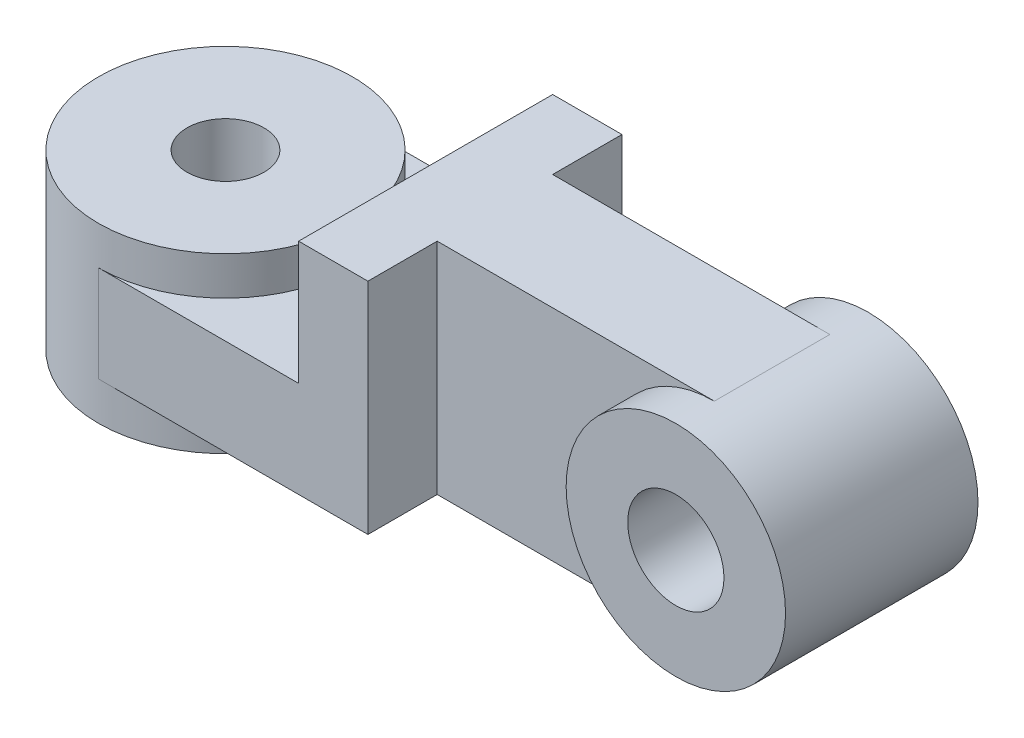
ISO-10303-21;
HEADER;
FILE_DESCRIPTION(('STEP AP214'),'2;1');
FILE_NAME('part.step','',(''),(''),'','','');
FILE_SCHEMA(('AUTOMOTIVE_DESIGN { 1 0 10303 214 1 1 1 1 }'));
ENDSEC;
DATA;
#1=APPLICATION_CONTEXT('core data for automotive mechanical design processes');
#2=APPLICATION_PROTOCOL_DEFINITION('international standard','automotive_design',2000,#1);
#3=PRODUCT_CONTEXT('',#1,'mechanical');
#4=PRODUCT('Part','Part','',(#3));
#5=PRODUCT_RELATED_PRODUCT_CATEGORY('part','',(#4));
#6=PRODUCT_DEFINITION_FORMATION('','',#4);
#7=PRODUCT_DEFINITION_CONTEXT('part definition',#1,'design');
#8=PRODUCT_DEFINITION('design','',#6,#7);
#9=PRODUCT_DEFINITION_SHAPE('','',#8);
#10=(LENGTH_UNIT() NAMED_UNIT(*) SI_UNIT(.MILLI.,.METRE.));
#11=(NAMED_UNIT(*) PLANE_ANGLE_UNIT() SI_UNIT($,.RADIAN.));
#12=(NAMED_UNIT(*) SI_UNIT($,.STERADIAN.) SOLID_ANGLE_UNIT());
#13=UNCERTAINTY_MEASURE_WITH_UNIT(LENGTH_MEASURE(1.E-05),#10,'distance_accuracy_value','');
#14=(GEOMETRIC_REPRESENTATION_CONTEXT(3) GLOBAL_UNCERTAINTY_ASSIGNED_CONTEXT((#13)) GLOBAL_UNIT_ASSIGNED_CONTEXT((#10,
#11,#12)) REPRESENTATION_CONTEXT('',''));
#15=CARTESIAN_POINT('',(0.,0.,0.));
#16=DIRECTION('',(0.,0.,1.));
#17=DIRECTION('',(1.,0.,0.));
#18=AXIS2_PLACEMENT_3D('',#15,#16,#17);
#19=CARTESIAN_POINT('',(70000.,12500.,-33000.));
#20=DIRECTION('',(-1.,0.,0.));
#21=DIRECTION('',(0.,0.,1.));
#22=AXIS2_PLACEMENT_3D('',#19,#20,#21);
#23=PLANE('',#22);
#24=DIRECTION('',(0.,1.,0.));
#25=VECTOR('',#24,1.);
#26=CARTESIAN_POINT('',(70000.,-12500.,-15000.));
#27=LINE('',#26,#25);
#28=CARTESIAN_POINT('',(70000.,-12500.,-15000.));
#29=VERTEX_POINT('',#28);
#30=CARTESIAN_POINT('',(70000.,44500.,-15000.));
#31=VERTEX_POINT('',#30);
#32=EDGE_CURVE('E152',#29,#31,#27,.T.);
#33=ORIENTED_EDGE('',*,*,#32,.F.);
#34=DIRECTION('',(0.,0.,-1.));
#35=VECTOR('',#34,1.);
#36=CARTESIAN_POINT('',(70000.,-12500.,-33000.));
#37=LINE('',#36,#35);
#38=CARTESIAN_POINT('',(70000.,-12500.,-33000.));
#39=VERTEX_POINT('',#38);
#40=EDGE_CURVE('E189',#29,#39,#37,.T.);
#41=ORIENTED_EDGE('',*,*,#40,.T.);
#42=DIRECTION('',(0.,-1.,0.));
#43=VECTOR('',#42,1.);
#44=CARTESIAN_POINT('',(70000.,12500.,-33000.));
#45=LINE('',#44,#43);
#46=CARTESIAN_POINT('',(70000.,44500.,-33000.));
#47=VERTEX_POINT('',#46);
#48=EDGE_CURVE('E191',#47,#39,#45,.T.);
#49=ORIENTED_EDGE('',*,*,#48,.F.);
#50=DIRECTION('',(0.,0.,-1.));
#51=VECTOR('',#50,1.);
#52=CARTESIAN_POINT('',(70000.,44500.,33000.));
#53=LINE('',#52,#51);
#54=EDGE_CURVE('E163',#31,#47,#53,.T.);
#55=ORIENTED_EDGE('',*,*,#54,.F.);
#56=EDGE_LOOP('',(#33,#41,#49,#55));
#57=FACE_BOUND('',#56,.T.);
#58=ADVANCED_FACE('F50',(#57),#23,.F.);
#59=CARTESIAN_POINT('',(0.,12500.,0.));
#60=DIRECTION('',(0.,1.,0.));
#61=DIRECTION('',(0.,0.,1.));
#62=AXIS2_PLACEMENT_3D('',#59,#60,#61);
#63=PLANE('',#62);
#64=DIRECTION('',(1.,0.,0.));
#65=VECTOR('',#64,1.);
#66=CARTESIAN_POINT('',(0.,12500.,33000.));
#67=LINE('',#66,#65);
#68=CARTESIAN_POINT('',(0.,12500.,33000.));
#69=VERTEX_POINT('',#68);
#70=CARTESIAN_POINT('',(52000.,12500.,33000.));
#71=VERTEX_POINT('',#70);
#72=EDGE_CURVE('E177',#69,#71,#67,.T.);
#73=ORIENTED_EDGE('',*,*,#72,.T.);
#74=DIRECTION('',(0.,0.,1.));
#75=VECTOR('',#74,1.);
#76=CARTESIAN_POINT('',(52000.,12500.,33000.));
#77=LINE('',#76,#75);
#78=CARTESIAN_POINT('',(52000.,12500.,-33000.));
#79=VERTEX_POINT('',#78);
#80=EDGE_CURVE('E67',#79,#71,#77,.T.);
#81=ORIENTED_EDGE('',*,*,#80,.F.);
#82=DIRECTION('',(-1.,0.,0.));
#83=VECTOR('',#82,1.);
#84=CARTESIAN_POINT('',(0.,12500.,-33000.));
#85=LINE('',#84,#83);
#86=CARTESIAN_POINT('',(-2.00982088115E-11,12500.,-33000.));
#87=VERTEX_POINT('',#86);
#88=EDGE_CURVE('E185',#79,#87,#85,.T.);
#89=ORIENTED_EDGE('',*,*,#88,.T.);
#90=CARTESIAN_POINT('',(0.,12500.,0.));
#91=DIRECTION('',(0.,-1.,0.));
#92=DIRECTION('',(0.,0.,1.));
#93=AXIS2_PLACEMENT_3D('',#90,#91,#92);
#94=CIRCLE('',#93,33000.);
#95=EDGE_CURVE('E176',#87,#69,#94,.T.);
#96=ORIENTED_EDGE('',*,*,#95,.T.);
#97=EDGE_LOOP('',(#73,#81,#89,#96));
#98=FACE_BOUND('',#97,.T.);
#99=ADVANCED_FACE('F233',(#98),#63,.T.);
#100=CARTESIAN_POINT('',(0.,22500.,0.));
#101=DIRECTION('',(0.,-1.,0.));
#102=DIRECTION('',(0.,0.,-1.));
#103=AXIS2_PLACEMENT_3D('',#100,#101,#102);
#104=CYLINDRICAL_SURFACE('',#103,33000.);
#105=DIRECTION('',(0.,-1.,0.));
#106=VECTOR('',#105,1.);
#107=CARTESIAN_POINT('',(0.,12500.,33000.));
#108=LINE('',#107,#106);
#109=CARTESIAN_POINT('',(0.,-12500.,33000.));
#110=VERTEX_POINT('',#109);
#111=EDGE_CURVE('E199',#69,#110,#108,.T.);
#112=ORIENTED_EDGE('',*,*,#111,.F.);
#113=ORIENTED_EDGE('',*,*,#95,.F.);
#114=DIRECTION('',(0.,-1.,0.));
#115=VECTOR('',#114,1.);
#116=CARTESIAN_POINT('',(0.,12500.,-33000.));
#117=LINE('',#116,#115);
#118=CARTESIAN_POINT('',(0.,-12500.,-33000.));
#119=VERTEX_POINT('',#118);
#120=EDGE_CURVE('E183',#87,#119,#117,.T.);
#121=ORIENTED_EDGE('',*,*,#120,.T.);
#122=CARTESIAN_POINT('',(0.,-12500.,0.));
#123=DIRECTION('',(0.,-1.,0.));
#124=DIRECTION('',(0.,0.,1.));
#125=AXIS2_PLACEMENT_3D('',#122,#123,#124);
#126=CIRCLE('',#125,33000.);
#127=EDGE_CURVE('E174',#119,#110,#126,.T.);
#128=ORIENTED_EDGE('',*,*,#127,.T.);
#129=EDGE_LOOP('',(#112,#113,#121,#128));
#130=FACE_BOUND('',#129,.T.);
#131=CARTESIAN_POINT('',(0.,22500.,0.));
#132=DIRECTION('',(0.,1.,0.));
#133=DIRECTION('',(0.,0.,1.));
#134=AXIS2_PLACEMENT_3D('',#131,#132,#133);
#135=CIRCLE('',#134,33000.);
#136=CARTESIAN_POINT('',(0.,22500.,33000.));
#137=VERTEX_POINT('',#136);
#138=EDGE_CURVE('E54',#137,#137,#135,.T.);
#139=ORIENTED_EDGE('',*,*,#138,.F.);
#140=EDGE_LOOP('',(#139));
#141=FACE_BOUND('',#140,.T.);
#142=CARTESIAN_POINT('',(0.,-22500.,0.));
#143=DIRECTION('',(0.,1.,0.));
#144=DIRECTION('',(0.,0.,1.));
#145=AXIS2_PLACEMENT_3D('',#142,#143,#144);
#146=CIRCLE('',#145,33000.);
#147=CARTESIAN_POINT('',(0.,-22500.,33000.));
#148=VERTEX_POINT('',#147);
#149=EDGE_CURVE('E210',#148,#148,#146,.T.);
#150=ORIENTED_EDGE('',*,*,#149,.T.);
#151=EDGE_LOOP('',(#150));
#152=FACE_BOUND('',#151,.T.);
#153=ADVANCED_FACE('F47',(#130,#141,#152),#104,.T.);
#154=CARTESIAN_POINT('',(0.,22500.,0.));
#155=DIRECTION('',(0.,1.,0.));
#156=DIRECTION('',(0.,0.,1.));
#157=AXIS2_PLACEMENT_3D('',#154,#155,#156);
#158=PLANE('',#157);
#159=CARTESIAN_POINT('',(0.,22500.,0.));
#160=DIRECTION('',(0.,1.,0.));
#161=DIRECTION('',(0.,0.,1.));
#162=AXIS2_PLACEMENT_3D('',#159,#160,#161);
#163=CIRCLE('',#162,10000.);
#164=CARTESIAN_POINT('',(0.,22500.,10000.));
#165=VERTEX_POINT('',#164);
#166=EDGE_CURVE('E203',#165,#165,#163,.T.);
#167=ORIENTED_EDGE('',*,*,#166,.F.);
#168=EDGE_LOOP('',(#167));
#169=FACE_BOUND('',#168,.T.);
#170=ORIENTED_EDGE('',*,*,#138,.T.);
#171=EDGE_LOOP('',(#170));
#172=FACE_BOUND('',#171,.T.);
#173=ADVANCED_FACE('F218',(#169,#172),#158,.T.);
#174=CARTESIAN_POINT('',(0.,-22500.,0.));
#175=DIRECTION('',(0.,1.,0.));
#176=DIRECTION('',(0.,0.,1.));
#177=AXIS2_PLACEMENT_3D('',#174,#175,#176);
#178=PLANE('',#177);
#179=CARTESIAN_POINT('',(0.,-22500.,0.));
#180=DIRECTION('',(0.,1.,0.));
#181=DIRECTION('',(0.,0.,1.));
#182=AXIS2_PLACEMENT_3D('',#179,#180,#181);
#183=CIRCLE('',#182,10000.);
#184=CARTESIAN_POINT('',(0.,-22500.,10000.));
#185=VERTEX_POINT('',#184);
#186=EDGE_CURVE('E202',#185,#185,#183,.T.);
#187=ORIENTED_EDGE('',*,*,#186,.T.);
#188=EDGE_LOOP('',(#187));
#189=FACE_BOUND('',#188,.T.);
#190=ORIENTED_EDGE('',*,*,#149,.F.);
#191=EDGE_LOOP('',(#190));
#192=FACE_BOUND('',#191,.T.);
#193=ADVANCED_FACE('F213',(#189,#192),#178,.F.);
#194=CARTESIAN_POINT('',(0.,-22500.,0.));
#195=DIRECTION('',(0.,1.,0.));
#196=DIRECTION('',(0.,0.,1.));
#197=AXIS2_PLACEMENT_3D('',#194,#195,#196);
#198=CYLINDRICAL_SURFACE('',#197,10000.);
#199=ORIENTED_EDGE('',*,*,#186,.F.);
#200=EDGE_LOOP('',(#199));
#201=FACE_BOUND('',#200,.T.);
#202=ORIENTED_EDGE('',*,*,#166,.T.);
#203=EDGE_LOOP('',(#202));
#204=FACE_BOUND('',#203,.T.);
#205=ADVANCED_FACE('F220',(#201,#204),#198,.F.);
#206=CARTESIAN_POINT('',(0.,12500.,33000.));
#207=DIRECTION('',(0.,0.,-1.));
#208=DIRECTION('',(-1.,0.,0.));
#209=AXIS2_PLACEMENT_3D('',#206,#207,#208);
#210=PLANE('',#209);
#211=DIRECTION('',(1.,0.,0.));
#212=VECTOR('',#211,1.);
#213=CARTESIAN_POINT('',(0.,-12500.,33000.));
#214=LINE('',#213,#212);
#215=CARTESIAN_POINT('',(70000.,-12500.,33000.));
#216=VERTEX_POINT('',#215);
#217=EDGE_CURVE('E187',#110,#216,#214,.T.);
#218=ORIENTED_EDGE('',*,*,#217,.T.);
#219=DIRECTION('',(0.,-1.,0.));
#220=VECTOR('',#219,1.);
#221=CARTESIAN_POINT('',(70000.,12500.,33000.));
#222=LINE('',#221,#220);
#223=CARTESIAN_POINT('',(70000.,44500.,33000.));
#224=VERTEX_POINT('',#223);
#225=EDGE_CURVE('E200',#224,#216,#222,.T.);
#226=ORIENTED_EDGE('',*,*,#225,.F.);
#227=DIRECTION('',(1.,0.,0.));
#228=VECTOR('',#227,1.);
#229=CARTESIAN_POINT('',(70000.,44500.,33000.));
#230=LINE('',#229,#228);
#231=CARTESIAN_POINT('',(52000.,44500.,33000.));
#232=VERTEX_POINT('',#231);
#233=EDGE_CURVE('E164',#232,#224,#230,.T.);
#234=ORIENTED_EDGE('',*,*,#233,.F.);
#235=DIRECTION('',(0.,-1.,0.));
#236=VECTOR('',#235,1.);
#237=CARTESIAN_POINT('',(52000.,44500.,33000.));
#238=LINE('',#237,#236);
#239=EDGE_CURVE('E166',#232,#71,#238,.T.);
#240=ORIENTED_EDGE('',*,*,#239,.T.);
#241=ORIENTED_EDGE('',*,*,#72,.F.);
#242=ORIENTED_EDGE('',*,*,#111,.T.);
#243=EDGE_LOOP('',(#218,#226,#234,#240,#241,#242));
#244=FACE_BOUND('',#243,.T.);
#245=ADVANCED_FACE('F222',(#244),#210,.F.);
#246=CARTESIAN_POINT('',(70000.,-12500.,15000.));
#247=VERTEX_POINT('',#246);
#248=EDGE_CURVE('E186',#216,#247,#37,.T.);
#249=ORIENTED_EDGE('',*,*,#248,.T.);
#250=DIRECTION('',(0.,1.,0.));
#251=VECTOR('',#250,1.);
#252=CARTESIAN_POINT('',(70000.,-12500.,15000.));
#253=LINE('',#252,#251);
#254=CARTESIAN_POINT('',(70000.,44500.,15000.));
#255=VERTEX_POINT('',#254);
#256=EDGE_CURVE('E145',#247,#255,#253,.T.);
#257=ORIENTED_EDGE('',*,*,#256,.T.);
#258=EDGE_CURVE('E160',#224,#255,#53,.T.);
#259=ORIENTED_EDGE('',*,*,#258,.F.);
#260=ORIENTED_EDGE('',*,*,#225,.T.);
#261=EDGE_LOOP('',(#249,#257,#259,#260));
#262=FACE_BOUND('',#261,.T.);
#263=ADVANCED_FACE('F234',(#262),#23,.F.);
#264=CARTESIAN_POINT('',(0.,12500.,-33000.));
#265=DIRECTION('',(0.,0.,1.));
#266=DIRECTION('',(1.,0.,0.));
#267=AXIS2_PLACEMENT_3D('',#264,#265,#266);
#268=PLANE('',#267);
#269=DIRECTION('',(-1.,0.,0.));
#270=VECTOR('',#269,1.);
#271=CARTESIAN_POINT('',(0.,-12500.,-33000.));
#272=LINE('',#271,#270);
#273=EDGE_CURVE('E179',#39,#119,#272,.T.);
#274=ORIENTED_EDGE('',*,*,#273,.T.);
#275=ORIENTED_EDGE('',*,*,#120,.F.);
#276=ORIENTED_EDGE('',*,*,#88,.F.);
#277=DIRECTION('',(0.,-1.,0.));
#278=VECTOR('',#277,1.);
#279=CARTESIAN_POINT('',(52000.,44500.,-33000.));
#280=LINE('',#279,#278);
#281=CARTESIAN_POINT('',(52000.,44500.,-33000.));
#282=VERTEX_POINT('',#281);
#283=EDGE_CURVE('E175',#282,#79,#280,.T.);
#284=ORIENTED_EDGE('',*,*,#283,.F.);
#285=DIRECTION('',(-1.,0.,0.));
#286=VECTOR('',#285,1.);
#287=CARTESIAN_POINT('',(70000.,44500.,-33000.));
#288=LINE('',#287,#286);
#289=EDGE_CURVE('E159',#47,#282,#288,.T.);
#290=ORIENTED_EDGE('',*,*,#289,.F.);
#291=ORIENTED_EDGE('',*,*,#48,.T.);
#292=EDGE_LOOP('',(#274,#275,#276,#284,#290,#291));
#293=FACE_BOUND('',#292,.T.);
#294=ADVANCED_FACE('F242',(#293),#268,.F.);
#295=CARTESIAN_POINT('',(0.,-12500.,0.));
#296=DIRECTION('',(0.,1.,0.));
#297=DIRECTION('',(0.,0.,1.));
#298=AXIS2_PLACEMENT_3D('',#295,#296,#297);
#299=PLANE('',#298);
#300=ORIENTED_EDGE('',*,*,#127,.F.);
#301=ORIENTED_EDGE('',*,*,#273,.F.);
#302=ORIENTED_EDGE('',*,*,#40,.F.);
#303=DIRECTION('',(-1.,0.,0.));
#304=VECTOR('',#303,1.);
#305=CARTESIAN_POINT('',(70000.,-12500.,-15000.));
#306=LINE('',#305,#304);
#307=CARTESIAN_POINT('',(142000.,-12500.,-15000.));
#308=VERTEX_POINT('',#307);
#309=EDGE_CURVE('E137',#308,#29,#306,.T.);
#310=ORIENTED_EDGE('',*,*,#309,.F.);
#311=DIRECTION('',(0.,0.,-1.));
#312=VECTOR('',#311,1.);
#313=CARTESIAN_POINT('',(142000.,-12500.,-15000.));
#314=LINE('',#313,#312);
#315=CARTESIAN_POINT('',(142000.,-12500.,15000.));
#316=VERTEX_POINT('',#315);
#317=EDGE_CURVE('E123',#316,#308,#314,.T.);
#318=ORIENTED_EDGE('',*,*,#317,.F.);
#319=DIRECTION('',(1.,0.,0.));
#320=VECTOR('',#319,1.);
#321=CARTESIAN_POINT('',(70000.,-12500.,15000.));
#322=LINE('',#321,#320);
#323=EDGE_CURVE('E136',#247,#316,#322,.T.);
#324=ORIENTED_EDGE('',*,*,#323,.F.);
#325=ORIENTED_EDGE('',*,*,#248,.F.);
#326=ORIENTED_EDGE('',*,*,#217,.F.);
#327=EDGE_LOOP('',(#300,#301,#302,#310,#318,#324,#325,#326));
#328=FACE_BOUND('',#327,.T.);
#329=ADVANCED_FACE('F132',(#328),#299,.F.);
#330=CARTESIAN_POINT('',(52000.,44500.,33000.));
#331=DIRECTION('',(1.,0.,0.));
#332=DIRECTION('',(0.,0.,-1.));
#333=AXIS2_PLACEMENT_3D('',#330,#331,#332);
#334=PLANE('',#333);
#335=ORIENTED_EDGE('',*,*,#80,.T.);
#336=ORIENTED_EDGE('',*,*,#239,.F.);
#337=DIRECTION('',(0.,0.,1.));
#338=VECTOR('',#337,1.);
#339=CARTESIAN_POINT('',(52000.,44500.,33000.));
#340=LINE('',#339,#338);
#341=EDGE_CURVE('E161',#282,#232,#340,.T.);
#342=ORIENTED_EDGE('',*,*,#341,.F.);
#343=ORIENTED_EDGE('',*,*,#283,.T.);
#344=EDGE_LOOP('',(#335,#336,#342,#343));
#345=FACE_BOUND('',#344,.T.);
#346=ADVANCED_FACE('F271',(#345),#334,.F.);
#347=CARTESIAN_POINT('',(0.,44500.,0.));
#348=DIRECTION('',(0.,1.,0.));
#349=DIRECTION('',(0.,0.,1.));
#350=AXIS2_PLACEMENT_3D('',#347,#348,#349);
#351=PLANE('',#350);
#352=ORIENTED_EDGE('',*,*,#258,.T.);
#353=DIRECTION('',(1.,0.,0.));
#354=VECTOR('',#353,1.);
#355=CARTESIAN_POINT('',(70000.,44500.,15000.));
#356=LINE('',#355,#354);
#357=CARTESIAN_POINT('',(142000.,44500.,15000.));
#358=VERTEX_POINT('',#357);
#359=EDGE_CURVE('E62',#255,#358,#356,.T.);
#360=ORIENTED_EDGE('',*,*,#359,.T.);
#361=DIRECTION('',(0.,0.,-1.));
#362=VECTOR('',#361,1.);
#363=CARTESIAN_POINT('',(142000.,44500.,-15000.));
#364=LINE('',#363,#362);
#365=CARTESIAN_POINT('',(142000.,44500.,-15000.));
#366=VERTEX_POINT('',#365);
#367=EDGE_CURVE('E129',#358,#366,#364,.T.);
#368=ORIENTED_EDGE('',*,*,#367,.T.);
#369=DIRECTION('',(-1.,0.,0.));
#370=VECTOR('',#369,1.);
#371=CARTESIAN_POINT('',(70000.,44500.,-15000.));
#372=LINE('',#371,#370);
#373=EDGE_CURVE('E141',#366,#31,#372,.T.);
#374=ORIENTED_EDGE('',*,*,#373,.T.);
#375=ORIENTED_EDGE('',*,*,#54,.T.);
#376=ORIENTED_EDGE('',*,*,#289,.T.);
#377=ORIENTED_EDGE('',*,*,#341,.T.);
#378=ORIENTED_EDGE('',*,*,#233,.T.);
#379=EDGE_LOOP('',(#352,#360,#368,#374,#375,#376,#377,#378));
#380=FACE_BOUND('',#379,.T.);
#381=ADVANCED_FACE('F268',(#380),#351,.T.);
#382=CARTESIAN_POINT('',(70000.,-12500.,-15000.));
#383=DIRECTION('',(0.,0.,-1.));
#384=DIRECTION('',(-1.,0.,0.));
#385=AXIS2_PLACEMENT_3D('',#382,#383,#384);
#386=PLANE('',#385);
#387=ORIENTED_EDGE('',*,*,#373,.F.);
#388=CARTESIAN_POINT('',(142000.,16000.,-15000.));
#389=DIRECTION('',(0.,0.,-1.));
#390=DIRECTION('',(-1.,0.,0.));
#391=AXIS2_PLACEMENT_3D('',#388,#389,#390);
#392=CIRCLE('',#391,28500.);
#393=EDGE_CURVE('E149',#366,#308,#392,.F.);
#394=ORIENTED_EDGE('',*,*,#393,.T.);
#395=ORIENTED_EDGE('',*,*,#309,.T.);
#396=ORIENTED_EDGE('',*,*,#32,.T.);
#397=EDGE_LOOP('',(#387,#394,#395,#396));
#398=FACE_BOUND('',#397,.T.);
#399=ADVANCED_FACE('F266',(#398),#386,.T.);
#400=CARTESIAN_POINT('',(70000.,-12500.,15000.));
#401=DIRECTION('',(0.,0.,1.));
#402=DIRECTION('',(1.,0.,0.));
#403=AXIS2_PLACEMENT_3D('',#400,#401,#402);
#404=PLANE('',#403);
#405=ORIENTED_EDGE('',*,*,#323,.T.);
#406=CARTESIAN_POINT('',(142000.,16000.,15000.));
#407=DIRECTION('',(0.,0.,1.));
#408=DIRECTION('',(1.,0.,0.));
#409=AXIS2_PLACEMENT_3D('',#406,#407,#408);
#410=CIRCLE('',#409,28500.);
#411=EDGE_CURVE('E11',#316,#358,#410,.F.);
#412=ORIENTED_EDGE('',*,*,#411,.T.);
#413=ORIENTED_EDGE('',*,*,#359,.F.);
#414=ORIENTED_EDGE('',*,*,#256,.F.);
#415=EDGE_LOOP('',(#405,#412,#413,#414));
#416=FACE_BOUND('',#415,.T.);
#417=ADVANCED_FACE('F142',(#416),#404,.T.);
#418=CARTESIAN_POINT('',(142000.,16000.,25000.));
#419=DIRECTION('',(0.,0.,-1.));
#420=DIRECTION('',(-1.,0.,0.));
#421=AXIS2_PLACEMENT_3D('',#418,#419,#420);
#422=CYLINDRICAL_SURFACE('',#421,28500.);
#423=ORIENTED_EDGE('',*,*,#393,.F.);
#424=ORIENTED_EDGE('',*,*,#367,.F.);
#425=ORIENTED_EDGE('',*,*,#411,.F.);
#426=ORIENTED_EDGE('',*,*,#317,.T.);
#427=EDGE_LOOP('',(#423,#424,#425,#426));
#428=FACE_BOUND('',#427,.T.);
#429=CARTESIAN_POINT('',(142000.,16000.,25000.));
#430=DIRECTION('',(0.,0.,1.));
#431=DIRECTION('',(1.,0.,0.));
#432=AXIS2_PLACEMENT_3D('',#429,#430,#431);
#433=CIRCLE('',#432,28500.);
#434=CARTESIAN_POINT('',(170500.,16000.,25000.));
#435=VERTEX_POINT('',#434);
#436=EDGE_CURVE('E315',#435,#435,#433,.T.);
#437=ORIENTED_EDGE('',*,*,#436,.F.);
#438=EDGE_LOOP('',(#437));
#439=FACE_BOUND('',#438,.T.);
#440=CARTESIAN_POINT('',(142000.,16000.,-25000.));
#441=DIRECTION('',(0.,0.,1.));
#442=DIRECTION('',(1.,0.,0.));
#443=AXIS2_PLACEMENT_3D('',#440,#441,#442);
#444=CIRCLE('',#443,28500.);
#445=CARTESIAN_POINT('',(170500.,16000.,-25000.));
#446=VERTEX_POINT('',#445);
#447=EDGE_CURVE('E307',#446,#446,#444,.T.);
#448=ORIENTED_EDGE('',*,*,#447,.T.);
#449=EDGE_LOOP('',(#448));
#450=FACE_BOUND('',#449,.T.);
#451=ADVANCED_FACE('F124',(#428,#439,#450),#422,.T.);
#452=CARTESIAN_POINT('',(142000.,16000.,25000.));
#453=DIRECTION('',(0.,0.,1.));
#454=DIRECTION('',(1.,0.,0.));
#455=AXIS2_PLACEMENT_3D('',#452,#453,#454);
#456=PLANE('',#455);
#457=CARTESIAN_POINT('',(142000.,16000.,25000.));
#458=DIRECTION('',(0.,0.,1.));
#459=DIRECTION('',(1.,0.,0.));
#460=AXIS2_PLACEMENT_3D('',#457,#458,#459);
#461=CIRCLE('',#460,12500.);
#462=CARTESIAN_POINT('',(154500.,16000.,25000.));
#463=VERTEX_POINT('',#462);
#464=EDGE_CURVE('E310',#463,#463,#461,.T.);
#465=ORIENTED_EDGE('',*,*,#464,.F.);
#466=EDGE_LOOP('',(#465));
#467=FACE_BOUND('',#466,.T.);
#468=ORIENTED_EDGE('',*,*,#436,.T.);
#469=EDGE_LOOP('',(#468));
#470=FACE_BOUND('',#469,.T.);
#471=ADVANCED_FACE('F288',(#467,#470),#456,.T.);
#472=CARTESIAN_POINT('',(142000.,16000.,-25000.));
#473=DIRECTION('',(0.,0.,1.));
#474=DIRECTION('',(1.,0.,0.));
#475=AXIS2_PLACEMENT_3D('',#472,#473,#474);
#476=PLANE('',#475);
#477=CARTESIAN_POINT('',(142000.,16000.,-25000.));
#478=DIRECTION('',(0.,0.,1.));
#479=DIRECTION('',(1.,0.,0.));
#480=AXIS2_PLACEMENT_3D('',#477,#478,#479);
#481=CIRCLE('',#480,12500.);
#482=CARTESIAN_POINT('',(154500.,16000.,-25000.));
#483=VERTEX_POINT('',#482);
#484=EDGE_CURVE('E302',#483,#483,#481,.T.);
#485=ORIENTED_EDGE('',*,*,#484,.T.);
#486=EDGE_LOOP('',(#485));
#487=FACE_BOUND('',#486,.T.);
#488=ORIENTED_EDGE('',*,*,#447,.F.);
#489=EDGE_LOOP('',(#488));
#490=FACE_BOUND('',#489,.T.);
#491=ADVANCED_FACE('F287',(#487,#490),#476,.F.);
#492=CARTESIAN_POINT('',(142000.,16000.,-25000.));
#493=DIRECTION('',(0.,0.,1.));
#494=DIRECTION('',(1.,0.,0.));
#495=AXIS2_PLACEMENT_3D('',#492,#493,#494);
#496=CYLINDRICAL_SURFACE('',#495,12500.);
#497=ORIENTED_EDGE('',*,*,#484,.F.);
#498=EDGE_LOOP('',(#497));
#499=FACE_BOUND('',#498,.T.);
#500=ORIENTED_EDGE('',*,*,#464,.T.);
#501=EDGE_LOOP('',(#500));
#502=FACE_BOUND('',#501,.T.);
#503=ADVANCED_FACE('F292',(#499,#502),#496,.F.);
#504=CLOSED_SHELL('',(#58,#99,#153,#173,#193,#205,#245,#263,#294,#329,#346,#381,#399,#417,#451,
#471,#491,#503));
#505=MANIFOLD_SOLID_BREP('B2',#504);
#506=ADVANCED_BREP_SHAPE_REPRESENTATION('',(#18,#505),#14);
#507=SHAPE_DEFINITION_REPRESENTATION(#9,#506);
ENDSEC;
END-ISO-10303-21;
